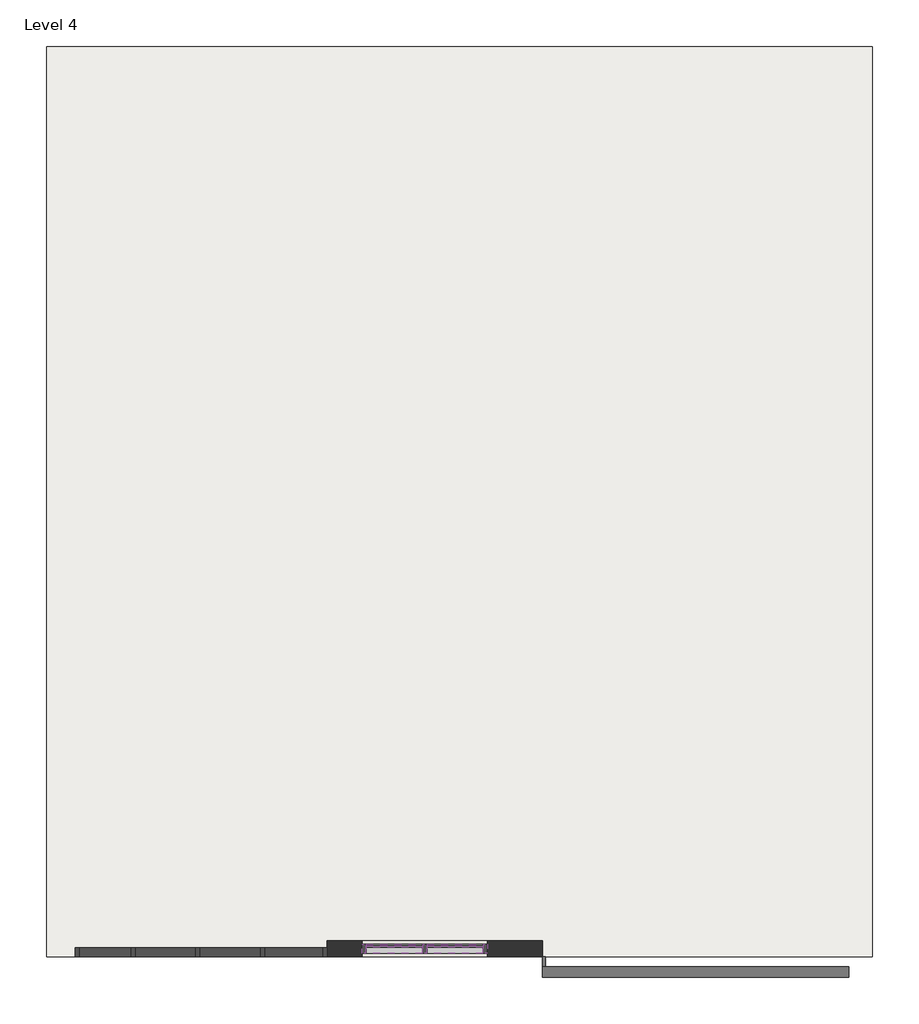
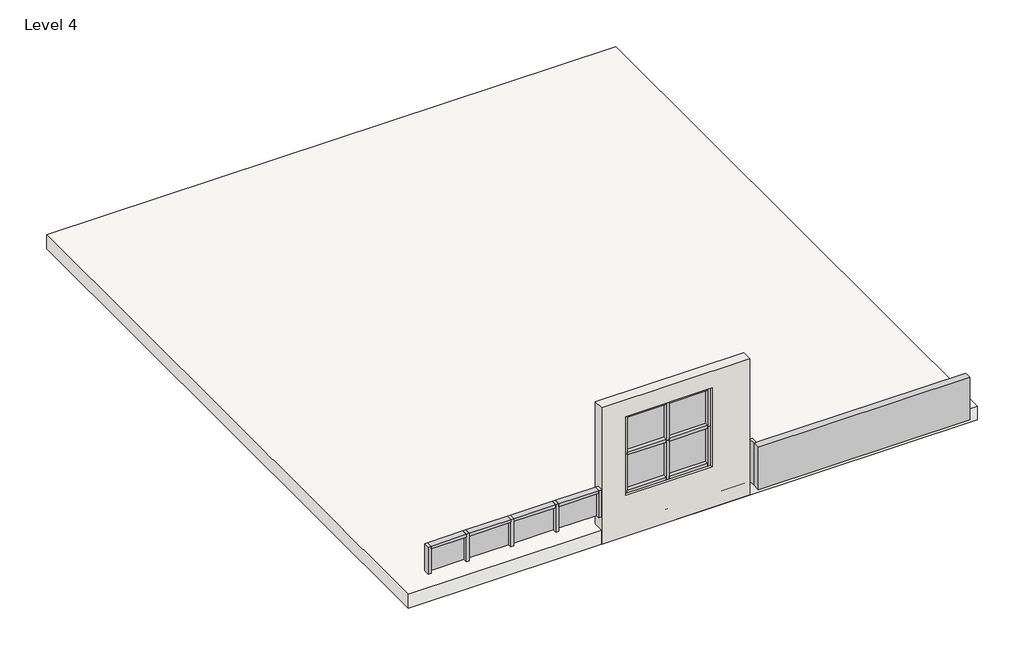
# One storey: 21 members, 8 plates, 2 proxies, 1 roof, 1 wall.
"""IFC4 building model written with IfcOpenShell, lengths in millimetres."""

from ifc_helpers import new_model, si_unit, frame, origin, place, context, project, spatial, polyline, outline, extrude, transform, mapped, element, save
from components import generic_models_5_generic_models_5_9fe8e222, generic_models_6_generic_models_6_594ef515, member_c17f1be2, member_ad567e07, member_b96be9f2, member_3ee5b9af, member_a908bda9, member_3a0a7659, member_4a8a2fe5, member_8834d53d, member_ceca9e34, system_panel_glazed_5425f88c, system_panel_glazed_fea38f3a, system_panel_glazed_a6f8d3da, system_panel_glazed_1cc9a2de

model = new_model("IFC4")

# Units and contexts
model_context = context("Model", 3, world=origin())
ifc_project = project(units=[si_unit("LENGTHUNIT", "METRE", prefix="MILLI")], contexts=[model_context])

# Site, building, storey
site = spatial("IfcSite", under=ifc_project)
building = spatial("IfcBuilding", under=site)
storey = spatial("IfcBuildingStorey", under=building, Name="Level 4", Elevation=9144.0)

# Proxies
placement = place(None, origin())
generic_models_5_generic_models_5_shape = generic_models_5_generic_models_5_9fe8e222(model_context)
element("IfcBuildingElementProxy", 1, Name="Generic Models 5 : Generic Models 5", ObjectType="Generic Models 5 : Generic Models 5", at=placement, inside=storey, context=model_context, shape_type="MappedRepresentation", body=[
    mapped(generic_models_5_generic_models_5_shape, transform((0.0, 0.0, 0.0), x_axis=(1.0, 0.0, 0.0), y_axis=(0.0, 1.0, 0.0), z_axis=(0.0, 0.0, 1.0))),
])
generic_models_6_generic_models_6_shape = generic_models_6_generic_models_6_594ef515(model_context)
element("IfcBuildingElementProxy", 2, Name="Generic Models 6 : Generic Models 6", ObjectType="Generic Models 6 : Generic Models 6", at=placement, inside=storey, context=model_context, shape_type="MappedRepresentation", body=[
    mapped(generic_models_6_generic_models_6_shape, transform((0.0, 0.0, 0.0), x_axis=(1.0, 0.0, 0.0), y_axis=(0.0, 1.0, 0.0), z_axis=(0.0, 0.0, 1.0))),
])

# Members
member_shape = member_c17f1be2(model_context)
element("IfcMember", 3, ObjectType="Rectangular Mullion : 2.5\" x 5\" rectangular", at=placement, inside=storey, context=model_context, shape_type="MappedRepresentation", body=[
    mapped(member_shape, transform((-14805.541855, -13739.8538163, 11818.3759079), x_axis=(0.0, 0.0, 1.0), y_axis=(0.0, -1.0, 0.0), z_axis=(1.0, 0.0, 0.0))),
])
element("IfcMember", 4, ObjectType="Rectangular Mullion : 2.5\" x 5\" rectangular", at=placement, inside=storey, context=model_context, shape_type="MappedRepresentation", body=[
    mapped(member_shape, transform((-13922.891855, -13739.8538163, 11818.3759079), x_axis=(0.0, 0.0, 1.0), y_axis=(0.0, -1.0, 0.0), z_axis=(1.0, 0.0, 0.0))),
])
member_2_shape = member_ad567e07(model_context)
element("IfcMember", 5, ObjectType="Rectangular Mullion : 2.5\" x 5\" rectangular", at=placement, inside=storey, context=model_context, shape_type="MappedRepresentation", body=[
    mapped(member_2_shape, transform((-13922.891855, -13739.8538163, 10938.1106834), x_axis=(0.0, 0.0, 1.0), y_axis=(0.0, -1.0, 0.0), z_axis=(1.0, 0.0, 0.0))),
])
element("IfcMember", 6, ObjectType="Rectangular Mullion : 2.5\" x 5\" rectangular", at=placement, inside=storey, context=model_context, shape_type="MappedRepresentation", body=[
    mapped(member_2_shape, transform((-14805.541855, -13739.8538163, 10938.1106834), x_axis=(0.0, 0.0, 1.0), y_axis=(0.0, -1.0, 0.0), z_axis=(1.0, 0.0, 0.0))),
])
element("IfcMember", 7, ObjectType="Rectangular Mullion : 2.5\" x 5\" rectangular", at=placement, inside=storey, context=model_context, shape_type="MappedRepresentation", body=[
    mapped(member_shape, transform((-14742.041855, -13739.8538163, 10057.845459), x_axis=(0.0, 0.0, -1.0), y_axis=(0.0, -1.0, 0.0), z_axis=(-1.0, 0.0, 0.0))),
])
element("IfcMember", 8, ObjectType="Rectangular Mullion : 2.5\" x 5\" rectangular", at=placement, inside=storey, context=model_context, shape_type="MappedRepresentation", body=[
    mapped(member_shape, transform((-15624.691855, -13739.8538163, 10057.845459), x_axis=(0.0, 0.0, -1.0), y_axis=(0.0, -1.0, 0.0), z_axis=(-1.0, 0.0, 0.0))),
])
member_3_shape = member_b96be9f2(model_context)
element("IfcMember", 9, ObjectType="Rectangular Mullion : 2.5\" x 5\" rectangular", at=placement, inside=storey, context=model_context, shape_type="MappedRepresentation", body=[
    mapped(member_3_shape, transform((-14773.791855, -13739.8538163, 10938.1106834), x_axis=(1.0, 0.0, 0.0), y_axis=(0.0, -1.0, 0.0), z_axis=(0.0, 0.0, -1.0))),
])
member_4_shape = member_3ee5b9af(model_context)
element("IfcMember", 10, ObjectType="Rectangular Mullion : 2.5\" x 5\" rectangular", at=placement, inside=storey, context=model_context, shape_type="MappedRepresentation", body=[
    mapped(member_4_shape, transform((-13859.391855, -13739.8538163, 10938.1106834), x_axis=(1.0, 0.0, 0.0), y_axis=(0.0, -1.0, 0.0), z_axis=(0.0, 0.0, -1.0))),
])
element("IfcMember", 11, ObjectType="Rectangular Mullion : 2.5\" x 5\" rectangular", at=placement, inside=storey, context=model_context, shape_type="MappedRepresentation", body=[
    mapped(member_3_shape, transform((-14773.791855, -13739.8538163, 10057.845459), x_axis=(1.0, 0.0, 0.0), y_axis=(0.0, -1.0, 0.0), z_axis=(0.0, 0.0, -1.0))),
])
element("IfcMember", 12, ObjectType="Rectangular Mullion : 2.5\" x 5\" rectangular", at=placement, inside=storey, context=model_context, shape_type="MappedRepresentation", body=[
    mapped(member_4_shape, transform((-13859.391855, -13739.8538163, 10057.845459), x_axis=(1.0, 0.0, 0.0), y_axis=(0.0, -1.0, 0.0), z_axis=(0.0, 0.0, -1.0))),
])
element("IfcMember", 13, ObjectType="Rectangular Mullion : 2.5\" x 5\" rectangular", at=placement, inside=storey, context=model_context, shape_type="MappedRepresentation", body=[
    mapped(member_4_shape, transform((-15688.191855, -13739.8538163, 10938.1106834), x_axis=(-1.0, 0.0, 0.0), y_axis=(0.0, -1.0, 0.0), z_axis=(0.0, 0.0, 1.0))),
])
element("IfcMember", 14, ObjectType="Rectangular Mullion : 2.5\" x 5\" rectangular", at=placement, inside=storey, context=model_context, shape_type="MappedRepresentation", body=[
    mapped(member_4_shape, transform((-15688.191855, -13739.8538163, 11818.3759079), x_axis=(-1.0, 0.0, 0.0), y_axis=(0.0, -1.0, 0.0), z_axis=(0.0, 0.0, 1.0))),
])
member_5_shape = member_a908bda9(model_context)
element("IfcMember", 15, ObjectType="Rectangular Mullion : 2.5\" x 5\" rectangular", at=placement, inside=storey, context=model_context, shape_type="MappedRepresentation", body=[
    mapped(member_5_shape, transform((-19866.491855, -13790.6538163, 10362.7538352), x_axis=(-1.0, 0.0, 0.0), y_axis=(0.0, -1.0, 0.0), z_axis=(0.0, 0.0, 1.0))),
])
member_6_shape = member_3a0a7659(model_context)
element("IfcMember", 16, ObjectType="Rectangular Mullion : 2.5\" x 5\" rectangular", at=placement, inside=storey, context=model_context, shape_type="MappedRepresentation", body=[
    mapped(member_6_shape, transform((-19060.041855, -13790.6538163, 10362.7538352), x_axis=(0.0, 0.0, 1.0), y_axis=(0.0, -1.0, 0.0), z_axis=(1.0, 0.0, 0.0))),
])
member_7_shape = member_4a8a2fe5(model_context)
element("IfcMember", 17, ObjectType="Rectangular Mullion : 2.5\" x 5\" rectangular", at=placement, inside=storey, context=model_context, shape_type="MappedRepresentation", body=[
    mapped(member_7_shape, transform((-19028.291855, -13790.6538163, 9753.6), x_axis=(1.0, 0.0, 0.0), y_axis=(0.0, -1.0, 0.0), z_axis=(0.0, 0.0, -1.0))),
])
element("IfcMember", 18, ObjectType="Rectangular Mullion : 2.5\" x 5\" rectangular", at=placement, inside=storey, context=model_context, shape_type="MappedRepresentation", body=[
    mapped(member_7_shape, transform((-18084.2585217, -13790.6538163, 9753.6), x_axis=(1.0, 0.0, 0.0), y_axis=(0.0, -1.0, 0.0), z_axis=(0.0, 0.0, -1.0))),
])
element("IfcMember", 19, ObjectType="Rectangular Mullion : 2.5\" x 5\" rectangular", at=placement, inside=storey, context=model_context, shape_type="MappedRepresentation", body=[
    mapped(member_7_shape, transform((-17140.2251883, -13790.6538163, 9753.6), x_axis=(1.0, 0.0, 0.0), y_axis=(0.0, -1.0, 0.0), z_axis=(0.0, 0.0, -1.0))),
])
member_8_shape = member_8834d53d(model_context)
element("IfcMember", 20, ObjectType="Rectangular Mullion : 2.5\" x 5\" rectangular", at=placement, inside=storey, context=model_context, shape_type="MappedRepresentation", body=[
    mapped(member_8_shape, transform((-17171.9751883, -13790.6538163, 10362.7538352), x_axis=(0.0, 0.0, 1.0), y_axis=(0.0, -1.0, 0.0), z_axis=(1.0, 0.0, 0.0))),
])
element("IfcMember", 21, ObjectType="Rectangular Mullion : 2.5\" x 5\" rectangular", at=placement, inside=storey, context=model_context, shape_type="MappedRepresentation", body=[
    mapped(member_8_shape, transform((-18116.0085217, -13790.6538163, 10362.7538352), x_axis=(0.0, 0.0, 1.0), y_axis=(0.0, -1.0, 0.0), z_axis=(1.0, 0.0, 0.0))),
])
member_9_shape = member_ceca9e34(model_context)
element("IfcMember", 22, ObjectType="Rectangular Mullion : 2.5\" x 5\" rectangular", at=placement, inside=storey, context=model_context, shape_type="MappedRepresentation", body=[
    mapped(member_9_shape, transform((-16259.691855, -13790.6538163, 10362.7538352), x_axis=(0.0, 0.0, 1.0), y_axis=(0.0, -1.0, 0.0), z_axis=(1.0, 0.0, 0.0))),
])
element("IfcMember", 23, ObjectType="Rectangular Mullion : 2.5\" x 5\" rectangular", at=placement, inside=storey, context=model_context, shape_type="MappedRepresentation", body=[
    mapped(member_5_shape, transform((-16196.191855, -13790.6538163, 9753.6), x_axis=(1.0, 0.0, 0.0), y_axis=(0.0, -1.0, 0.0), z_axis=(0.0, 0.0, -1.0))),
])

# Plates
system_panel_glazed_shape = system_panel_glazed_5425f88c(model_context)
element("IfcPlate", 24, ObjectType="System Panel : Glazed", at=placement, inside=storey, context=model_context, shape_type="MappedRepresentation", body=[
    mapped(system_panel_glazed_shape, transform((-15215.116855, -13739.8538163, 10121.345459), x_axis=(1.0, 0.0, 0.0), y_axis=(0.0, 1.0, 0.0), z_axis=(0.0, 0.0, 1.0))),
])
element("IfcPlate", 25, ObjectType="System Panel : Glazed", at=placement, inside=storey, context=model_context, shape_type="MappedRepresentation", body=[
    mapped(system_panel_glazed_shape, transform((-14332.466855, -13739.8538163, 10121.345459), x_axis=(1.0, 0.0, 0.0), y_axis=(0.0, 1.0, 0.0), z_axis=(0.0, 0.0, 1.0))),
])
element("IfcPlate", 26, ObjectType="System Panel : Glazed", at=placement, inside=storey, context=model_context, shape_type="MappedRepresentation", body=[
    mapped(system_panel_glazed_shape, transform((-15215.116855, -13739.8538163, 10969.8606834), x_axis=(1.0, 0.0, 0.0), y_axis=(0.0, 1.0, 0.0), z_axis=(0.0, 0.0, 1.0))),
])
element("IfcPlate", 27, ObjectType="System Panel : Glazed", at=placement, inside=storey, context=model_context, shape_type="MappedRepresentation", body=[
    mapped(system_panel_glazed_shape, transform((-14332.466855, -13739.8538163, 10969.8606834), x_axis=(1.0, 0.0, 0.0), y_axis=(0.0, 1.0, 0.0), z_axis=(0.0, 0.0, 1.0))),
])
system_panel_glazed_2_shape = system_panel_glazed_fea38f3a(model_context)
element("IfcPlate", 28, ObjectType="System Panel : Glazed", at=placement, inside=storey, context=model_context, shape_type="MappedRepresentation", body=[
    mapped(system_panel_glazed_2_shape, transform((-19431.516855, -13790.6538163, 9753.6), x_axis=(1.0, 0.0, 0.0), y_axis=(0.0, 1.0, 0.0), z_axis=(0.0, 0.0, 1.0))),
])
system_panel_glazed_3_shape = system_panel_glazed_a6f8d3da(model_context)
element("IfcPlate", 29, ObjectType="System Panel : Glazed", at=placement, inside=storey, context=model_context, shape_type="MappedRepresentation", body=[
    mapped(system_panel_glazed_3_shape, transform((-18556.2751883, -13790.6538163, 9753.6), x_axis=(1.0, 0.0, 0.0), y_axis=(0.0, 1.0, 0.0), z_axis=(0.0, 0.0, 1.0))),
])
element("IfcPlate", 30, ObjectType="System Panel : Glazed", at=placement, inside=storey, context=model_context, shape_type="MappedRepresentation", body=[
    mapped(system_panel_glazed_3_shape, transform((-17612.241855, -13790.6538163, 9753.6), x_axis=(1.0, 0.0, 0.0), y_axis=(0.0, 1.0, 0.0), z_axis=(0.0, 0.0, 1.0))),
])
system_panel_glazed_4_shape = system_panel_glazed_1cc9a2de(model_context)
element("IfcPlate", 31, ObjectType="System Panel : Glazed", at=placement, inside=storey, context=model_context, shape_type="MappedRepresentation", body=[
    mapped(system_panel_glazed_4_shape, transform((-16684.0835217, -13790.6538163, 9753.6), x_axis=(1.0, 0.0, 0.0), y_axis=(0.0, 1.0, 0.0), z_axis=(0.0, 0.0, 1.0))),
])

# Roof
element("IfcRoof", 32, ObjectType="Generic - 12\"", at=placement, inside=storey, context=model_context, shape_type="SweptSolid", body=[
    extrude(outline(polyline([(-20285.591855, -595.3538163), (-8245.991855, -595.3538163), (-8245.991855, -13854.1538163), (-20285.591855, -13854.1538163), (-20285.591855, -595.3538163)])), frame((0.0, 0.0, 9144.0), z_axis=(0.0, 0.0, 1.0), x_axis=(1.0, 0.0, 0.0)), (0.0, 0.0, 1.0), 304.8),
])

# Wall
element("IfcWall", 33, ObjectType="9\"", at=placement, inside=storey, context=model_context, shape_type="SweptSolid", body=[
    extrude(outline(polyline([(9144.0, -16196.191855), (9144.0, -13059.291855), (12192.0, -13059.291855), (12192.0, -16196.191855), (9144.0, -16196.191855)]), holes=[polyline([(10057.845459, -15688.191855), (11818.3759079, -15688.191855), (11818.3759079, -13859.391855), (10057.845459, -13859.391855), (10057.845459, -15688.191855)])]), frame((0.0, -13854.1538163, 0.0), z_axis=(0.0, 1.0, 0.0), x_axis=(0.0, 0.0, 1.0)), (0.0, 0.0, 1.0), 228.6),
])

save(model, "model.ifc")

# Revit data of these elements
# Type "Rectangular Mullion : 2.5\" x 5\" rectangular"
#   built-in parameter 1007304 = 0.416667 (stored number, unit not read)
#   built-in parameter 1007301 = 0.104167 (stored number, unit not read)
#   built-in parameter 1007300 = 0.104167 (stored number, unit not read)
# Type "System Panel : Glazed"
#   Construction Type Id = "GSP4R"
#   Analytic Construction = "1/8 in Pilkington single glazing"
#   Visual Light Transmittance = 0.9
#   Solar Heat Gain Coefficient = 0.86
#   Heat Transfer Coefficient (U) = 1.18115 BTU/(h·ft²·°F)
#   Define Thermal Properties by = 1
# Type "Generic - 12\""
#   Assembly Code = "B1020"
#   Layers, outside or top first: 1' - 0" no material (function 1)
# Type "9\""
#   Assembly Code = "B2010"
#   Layers, outside or top first: 0' - 9" no material (function 1)
# Element 1 (IfcBuildingElementProxy, "Generic Models 5 : Generic Models 5")
#   Phase Created = New Construction
# Element 2 (IfcBuildingElementProxy, "Generic Models 6 : Generic Models 6")
#   Phase Created = New Construction
# Elements 3, 4, 5, 6, 7, 8, 9, 10, 11, 12, 13, 14, 15, 16, 17, 18, 19, 20, 21, 22, 23 (IfcMember, "Rectangular Mullion : 2.5\" x 5\" rectangular")
#   Phase Created = New Construction
#   Materials on its faces: "Aluminum"
# Elements 24, 25, 26, 27, 28, 29, 30, 31 (IfcPlate, "System Panel : Glazed")
#   Phase Created = New Construction
#   Materials on its faces: "Glass"
# Element 32 (IfcRoof, "Generic - 12\"")
#   built-in parameter 1001705 = 31 (stored number, unit not read)
#   built-in parameter 1001710 = 33615
#   Phase Created = New Construction
#   Materials on its faces: "Default Roof"
# Element 33 (IfcWall, "9\"")
#   Top Offset = 0' - 0"
#   Base Offset = 0' - 0"
#   Unconnected Height = 10' - 0"
#   wall height = 10' - 0"
#   Phase Created = New Construction
#   Base Constraint = Level 4
#   Materials on its faces: "Default Wall"
# Materials
#   "Aluminum": class "Metal", colour RGB 247 247 247, transparency 0, Description = "Aluminum 6061", Cost = 0
#   "Glass": class "Glass", colour RGB 0 128 192, transparency 0.75, Description = "Soda Lime Glass", Cost = 0
#   "Default Roof": colour RGB 88 101 114, transparency 0, Cost = 0
#   "Default Wall": colour RGB 128 128 128, transparency 0, Cost = 0
